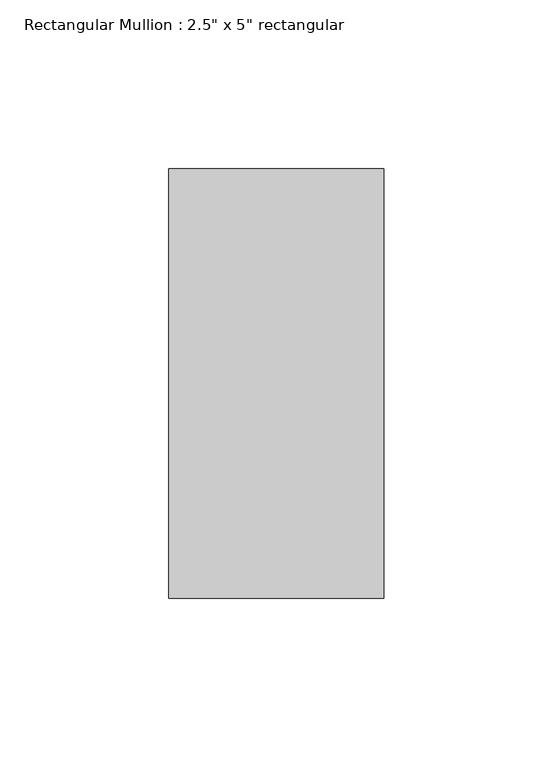
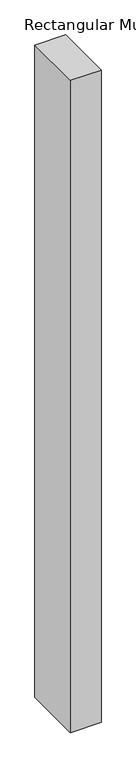
"""IFC4 building model written with IfcOpenShell, lengths in millimetres: member geometry."""

from ifc_helpers import new_model, si_unit, frame, origin, place, context, project, spatial, polyline, outline, extrude, source, transform, mapped, element, save


def member_041bc147(model_context):
    return source(origin(), model_context, "Body", "SweptSolid", [
        extrude(outline(polyline([(0.0, 63.5), (0.0, -63.5), (-63.5, -63.5), (-63.5, 63.5), (0.0, 63.5)])), frame((0.0, 0.0, -1428.2525568), z_axis=(0.0, 0.0, 1.0), x_axis=(1.0, 0.0, 0.0)), (0.0, 0.0, 1.0), 1428.2525568),
    ])


if __name__ == "__main__":
    model = new_model("IFC4")
    model_context = context("Model", 3, world=origin())
    ifc_project = project(units=[si_unit("LENGTHUNIT", "METRE", prefix="MILLI")], contexts=[model_context])
    site = spatial("IfcSite", under=ifc_project)
    building = spatial("IfcBuilding", under=site)
    placement = place(None, origin())
    member_shape = member_041bc147(model_context)
    element("IfcMember", 1, ObjectType="Rectangular Mullion : 2.5\" x 5\" rectangular", at=placement, inside=building, context=model_context, shape_type="MappedRepresentation", body=[
        mapped(member_shape, transform((0.0, 0.0, 0.0), x_axis=(1.0, 0.0, 0.0), y_axis=(0.0, 1.0, 0.0), z_axis=(0.0, 0.0, 1.0))),
    ])
    save(model, "model.ifc")

# Revit data of these elements
# Type "Rectangular Mullion : 2.5\" x 5\" rectangular"
#   built-in parameter 1007304 = 0.416667 (stored number, unit not read)
#   built-in parameter 1007301 = 0.104167 (stored number, unit not read)
#   built-in parameter 1007300 = 0.104167 (stored number, unit not read)
# Element 1 (IfcMember, "Rectangular Mullion : 2.5\" x 5\" rectangular")
#   Materials on its faces: "Aluminum"
# Materials
#   "Aluminum": class "Metal", colour RGB 247 247 247, transparency 0, Description = "Aluminum 6061", Cost = 0
